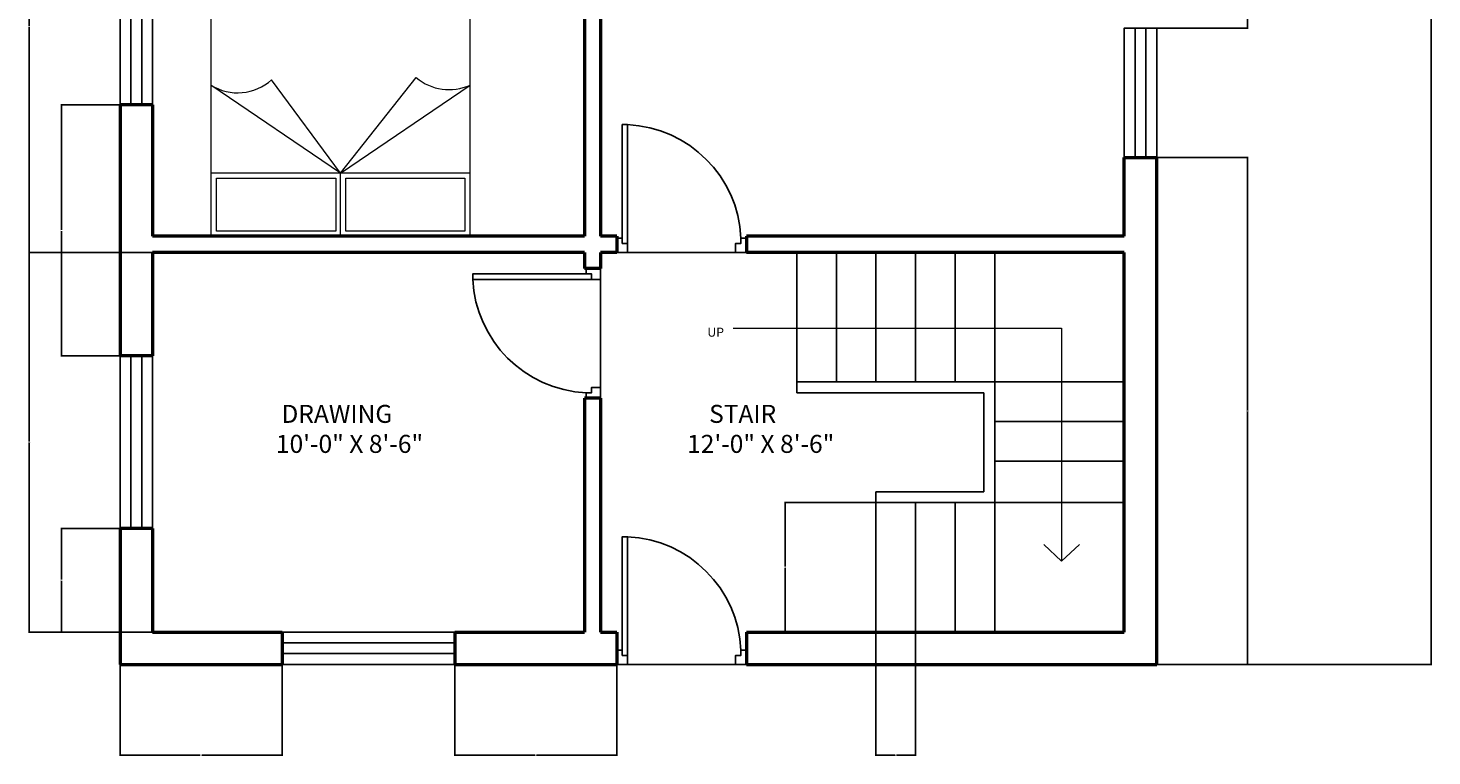
# Model space of a CAD drawing. Units: inches. Extents: x 17078 to 17468, y 5298 to 5853.
# Tile 1 of 3: x 17078 to 17468, y 5298 to 5500. Entities that reach past the tile are written whole.
import ezdxf

# ---------------------------------------------------------------- set-up
doc = ezdxf.new("R2010")
doc.units = ezdxf.units.IN
for name, color, linetype, lineweight in [('A-ANNO-DIMS', 2, 'Continuous', 18), ('A-ANNO-SYMB', 7, 'Continuous', 18), ('A-ANNO-TEXT', 7, 'Continuous', 18), ('A-AREA-IDEN', 7, 'Continuous', 18), ('door', 30, 'Continuous', 25), ('furniture', 9, 'Continuous', 18), ('Staircase', 11, 'Continuous', 25), ('wall', 7, 'Continuous', 50), ('window1', 151, 'Continuous', 25)]:
    doc.layers.add(name, color=color, linetype=linetype, lineweight=lineweight)
doc.styles.get("Standard").update_dxf_attribs({"font": 'arial.ttf'})
doc.dimstyles.get("Standard").update_dxf_attribs({"dimtxt": 0.18, "dimasz": 0.18, "dimexe": 0.18, "dimexo": 0.0625, "dimgap": 0.09, "dimtad": 0, "dimtih": 1, "dimtoh": 1, "dimdec": 4, "dimzin": 0, "dimdsep": 46, "dimtxsty": 'Standard', "dimcen": 0.09, "dimadec": 0, "dimazin": 0, "dimtfac": 1, "dimtdec": 4, "dimtofl": 0, "dimtmove": 0, "dimatfit": 3, "dimfxl": 1, "dimtolj": 1, "dimtzin": 0, "dimarcsym": 0})

# ---------------------------------------------------------------- blocks, each defined once
blk = doc.blocks.new('w2')
at = {"layer": 'window1'}
for p, q in [((17539.72, 5675.98), (17539.72, 5627.98)), ((17542.72, 5675.98), (17542.72, 5627.98))]:
    blk.add_line(p, q, dxfattribs=at)
blk.add_lwpolyline([(17536.72, 5627.98), (17545.72, 5627.98), (17545.72, 5675.98), (17536.72, 5675.98)], close=True, dxfattribs=at)
blk = doc.blocks.new('w1')
at = {"layer": 'window1'}
for p, q in [((17477.6, 5616.65), (17477.6, 5580.65)), ((17480.6, 5616.65), (17480.6, 5580.65))]:
    blk.add_line(p, q, dxfattribs=at)
blk.add_lwpolyline([(17474.6, 5580.65), (17483.6, 5580.65), (17483.6, 5616.65), (17474.6, 5616.65)], close=True, dxfattribs=at)
blk = doc.blocks.new('d1')
at = {"layer": 'door'}
blk.add_line((17631.7, 5593.67), (17667.7, 5593.67), dxfattribs=at)
blk.add_lwpolyline([(17633.2, 5596.17), (17634.7, 5596.17), (17634.7, 5629.17), (17633.2, 5629.17)], close=True, dxfattribs=at)
for points in [[(17634.7, 5593.67), (17631.7, 5593.67), (17631.7, 5597.67), (17633.2, 5597.67), (17633.2, 5596.17), (17634.7, 5596.17), (17634.7, 5593.67)], [(17664.7, 5593.67), (17667.7, 5593.67), (17667.7, 5597.67), (17666.2, 5597.67), (17666.2, 5596.17), (17664.7, 5596.17), (17664.7, 5593.67)]]:
    blk.add_lwpolyline(points, dxfattribs=at)
blk.add_arc((17633.2, 5596.17), 33.03, 2.6026, 87.3974, dxfattribs=at)
blk = doc.blocks.new('BED')
at = {"layer": 'furniture'}
for p, q in [((17631.72, 5825.16), (17631.72, 5807.64)), ((17595.72, 5807.64), (17667.72, 5807.64)), ((17631.72, 5807.64), (17595.72, 5783.16)), ((17631.72, 5807.64), (17610.71, 5781.09)), ((17631.72, 5807.64), (17667.72, 5783.16)), ((17631.72, 5807.64), (17650.87, 5781.67))]:
    blk.add_line(p, q, dxfattribs=at)
for points in [[(17595.72, 5741.16), (17667.72, 5741.16), (17667.72, 5825.16), (17595.72, 5825.16)], [(17597.14, 5823.74), (17630.27, 5823.74), (17630.27, 5809), (17597.14, 5809)], [(17633.01, 5823.74), (17666.14, 5823.74), (17666.14, 5809), (17633.01, 5809)]]:
    blk.add_lwpolyline(points, close=True, dxfattribs=at)
for centre, radius, start, end in [((17601.58, 5770.29), 14.15, 49.7949, 114.4561), ((17660.27, 5771.38), 13.94, 57.7012, 132.4176)]:
    blk.add_arc(centre, radius, start, end, dxfattribs=at)
blk = doc.blocks.new('*D22')
at = {"layer": 'A-ANNO-DIMS', "color": 0, "lineweight": -2, "transparency": 16777216}
for p, q in [((17391.6, 5827.52), (17467.96, 5827.52)), ((17467.78, 5827.34), (17467.78, 5575.7)), ((17467.78, 5323.7), (17467.78, 5575.34)), ((17391.6, 5323.52), (17467.96, 5323.52))]:
    blk.add_line(p, q, dxfattribs=at)
at = {"layer": 'A-ANNO-DIMS', "color": 0, "transparency": 16777216}
for points in [[(17467.75, 5827.34), (17467.81, 5827.34), (17467.78, 5827.52)], [(17467.75, 5323.7), (17467.81, 5323.7), (17467.78, 5323.52)]]:
    blk.add_solid(points, dxfattribs=at)
at = {"layer": 'Defpoints', "color": 0, "transparency": 16777216}
for p in [(17391.53, 5827.52), (17467.78, 5827.52), (17391.53, 5323.52)]:
    blk.add_point(p, dxfattribs=at)
at = {"layer": 'A-ANNO-DIMS', "color": 0, "transparency": 16777216, "insert": (17467.78, 5575.52), "char_height": 0.18, "attachment_point": 5}
blk.add_mtext('\\A1;504', dxfattribs=at)
blk = doc.blocks.new('*D23')
at = {"layer": 'A-ANNO-DIMS', "color": 0, "lineweight": -2, "transparency": 16777216}
for p, q in [((17112.47, 5438.02), (17078.1, 5438.02)), ((17078.28, 5437.84), (17078.28, 5385.45)), ((17078.28, 5332.7), (17078.28, 5385.09)), ((17112.47, 5332.52), (17078.1, 5332.52))]:
    blk.add_line(p, q, dxfattribs=at)
at = {"layer": 'A-ANNO-DIMS', "color": 0, "transparency": 16777216}
for points in [[(17078.25, 5437.84), (17078.31, 5437.84), (17078.28, 5438.02)], [(17078.25, 5332.7), (17078.31, 5332.7), (17078.28, 5332.52)]]:
    blk.add_solid(points, dxfattribs=at)
at = {"layer": 'Defpoints', "color": 0, "transparency": 16777216}
for p in [(17078.28, 5438.02), (17112.53, 5438.02), (17112.53, 5332.52)]:
    blk.add_point(p, dxfattribs=at)
at = {"layer": 'A-ANNO-DIMS', "color": 0, "transparency": 16777216, "insert": (17078.28, 5385.27), "char_height": 0.18, "attachment_point": 5}
blk.add_mtext('\\A1;105.5', dxfattribs=at)
blk = doc.blocks.new('*D24')
at = {"layer": 'A-ANNO-DIMS', "color": 0, "lineweight": -2, "transparency": 16777216}
for p, q in [((17112.47, 5563.52), (17078.1, 5563.52)), ((17078.28, 5563.34), (17078.28, 5500.95)), ((17078.28, 5438.2), (17078.28, 5500.59)), ((17112.47, 5438.02), (17078.1, 5438.02))]:
    blk.add_line(p, q, dxfattribs=at)
at = {"layer": 'A-ANNO-DIMS', "color": 0, "transparency": 16777216}
for points in [[(17078.25, 5563.34), (17078.31, 5563.34), (17078.28, 5563.52)], [(17078.25, 5438.2), (17078.31, 5438.2), (17078.28, 5438.02)]]:
    blk.add_solid(points, dxfattribs=at)
at = {"layer": 'Defpoints', "color": 0, "transparency": 16777216}
for p in [(17078.28, 5563.52), (17112.53, 5563.52), (17112.53, 5438.02)]:
    blk.add_point(p, dxfattribs=at)
at = {"layer": 'A-ANNO-DIMS', "color": 0, "transparency": 16777216, "insert": (17078.28, 5500.77), "char_height": 0.18, "attachment_point": 5}
blk.add_mtext('\\A1;125.5', dxfattribs=at)
blk = doc.blocks.new('*D26')
at = {"layer": 'A-ANNO-DIMS', "color": 0, "lineweight": -2, "transparency": 16777216}
for p, q in [((17103.53, 5323.46), (17103.53, 5298.09)), ((17148.53, 5323.46), (17148.53, 5298.09)), ((17103.71, 5298.27), (17125.81, 5298.27)), ((17148.35, 5298.27), (17126.26, 5298.27))]:
    blk.add_line(p, q, dxfattribs=at)
at = {"layer": 'A-ANNO-DIMS', "color": 0, "transparency": 16777216}
for points in [[(17103.71, 5298.3), (17103.71, 5298.24), (17103.53, 5298.27)], [(17148.35, 5298.3), (17148.35, 5298.24), (17148.53, 5298.27)]]:
    blk.add_solid(points, dxfattribs=at)
at = {"layer": 'Defpoints', "color": 0, "transparency": 16777216}
for p in [(17103.53, 5323.52), (17148.53, 5323.52), (17148.53, 5298.27)]:
    blk.add_point(p, dxfattribs=at)
at = {"layer": 'A-ANNO-DIMS', "color": 0, "transparency": 16777216, "insert": (17126.03, 5298.27), "char_height": 0.18, "attachment_point": 5}
blk.add_mtext('\\A1;45', dxfattribs=at)
blk = doc.blocks.new('*D27')
at = {"layer": 'A-ANNO-DIMS', "color": 0, "lineweight": -2, "transparency": 16777216}
for p, q in [((17196.53, 5323.46), (17196.53, 5298.09)), ((17241.53, 5323.46), (17241.53, 5298.09)), ((17196.71, 5298.27), (17218.81, 5298.27)), ((17241.35, 5298.27), (17219.26, 5298.27))]:
    blk.add_line(p, q, dxfattribs=at)
at = {"layer": 'A-ANNO-DIMS', "color": 0, "transparency": 16777216}
for points in [[(17196.71, 5298.3), (17196.71, 5298.24), (17196.53, 5298.27)], [(17241.35, 5298.3), (17241.35, 5298.24), (17241.53, 5298.27)]]:
    blk.add_solid(points, dxfattribs=at)
at = {"layer": 'Defpoints', "color": 0, "transparency": 16777216}
for p in [(17196.53, 5323.52), (17241.53, 5323.52), (17241.53, 5298.27)]:
    blk.add_point(p, dxfattribs=at)
at = {"layer": 'A-ANNO-DIMS', "color": 0, "transparency": 16777216, "insert": (17219.03, 5298.27), "char_height": 0.18, "attachment_point": 5}
blk.add_mtext('\\A1;45', dxfattribs=at)
blk = doc.blocks.new('*D28')
at = {"layer": 'A-ANNO-DIMS', "color": 0, "lineweight": -2, "transparency": 16777216}
for p, q in [((17112.47, 5361.27), (17087.1, 5361.27)), ((17087.28, 5361.09), (17087.28, 5347.08)), ((17087.28, 5332.7), (17087.28, 5346.71)), ((17112.47, 5332.52), (17087.1, 5332.52))]:
    blk.add_line(p, q, dxfattribs=at)
at = {"layer": 'A-ANNO-DIMS', "color": 0, "transparency": 16777216}
for points in [[(17087.25, 5361.09), (17087.31, 5361.09), (17087.28, 5361.27)], [(17087.25, 5332.7), (17087.31, 5332.7), (17087.28, 5332.52)]]:
    blk.add_solid(points, dxfattribs=at)
at = {"layer": 'Defpoints', "color": 0, "transparency": 16777216}
for p in [(17087.28, 5361.27), (17112.53, 5361.27), (17112.53, 5332.52)]:
    blk.add_point(p, dxfattribs=at)
at = {"layer": 'A-ANNO-DIMS', "color": 0, "transparency": 16777216, "insert": (17087.28, 5346.9), "char_height": 0.18, "attachment_point": 5}
blk.add_mtext('\\A1;28.75', dxfattribs=at)
blk = doc.blocks.new('*D29')
at = {"layer": 'A-ANNO-DIMS', "color": 0, "lineweight": -2, "transparency": 16777216}
for p, q in [((17112.47, 5479.02), (17087.1, 5479.02)), ((17087.28, 5478.84), (17087.28, 5444.33)), ((17087.28, 5409.45), (17087.28, 5443.96)), ((17112.47, 5409.27), (17087.1, 5409.27))]:
    blk.add_line(p, q, dxfattribs=at)
at = {"layer": 'A-ANNO-DIMS', "color": 0, "transparency": 16777216}
for points in [[(17087.25, 5478.84), (17087.31, 5478.84), (17087.28, 5479.02)], [(17087.25, 5409.45), (17087.31, 5409.45), (17087.28, 5409.27)]]:
    blk.add_solid(points, dxfattribs=at)
at = {"layer": 'Defpoints', "color": 0, "transparency": 16777216}
for p in [(17087.28, 5479.02), (17112.53, 5479.02), (17112.53, 5409.27)]:
    blk.add_point(p, dxfattribs=at)
at = {"layer": 'A-ANNO-DIMS', "color": 0, "transparency": 16777216, "insert": (17087.28, 5444.15), "char_height": 0.18, "attachment_point": 5}
blk.add_mtext('\\A1;69.75', dxfattribs=at)
blk = doc.blocks.new('*D32')
at = {"layer": 'A-ANNO-DIMS', "color": 0, "lineweight": -2, "transparency": 16777216}
for p, q in [((17391.6, 5464.35), (17416.96, 5464.35)), ((17416.78, 5464.17), (17416.78, 5394.12)), ((17416.78, 5323.7), (17416.78, 5393.76)), ((17391.6, 5323.52), (17416.96, 5323.52))]:
    blk.add_line(p, q, dxfattribs=at)
at = {"layer": 'A-ANNO-DIMS', "color": 0, "transparency": 16777216}
for points in [[(17416.75, 5464.17), (17416.81, 5464.17), (17416.78, 5464.35)], [(17416.75, 5323.7), (17416.81, 5323.7), (17416.78, 5323.52)]]:
    blk.add_solid(points, dxfattribs=at)
at = {"layer": 'Defpoints', "color": 0, "transparency": 16777216}
for p in [(17391.53, 5464.35), (17391.53, 5323.52), (17416.78, 5323.52)]:
    blk.add_point(p, dxfattribs=at)
at = {"layer": 'A-ANNO-DIMS', "color": 0, "transparency": 16777216, "insert": (17416.78, 5393.94), "char_height": 0.18, "attachment_point": 5}
blk.add_mtext('\\A1;140.83', dxfattribs=at)
blk = doc.blocks.new('*D33')
at = {"layer": 'A-ANNO-DIMS', "color": 0, "lineweight": -2, "transparency": 16777216}
for p, q in [((17391.6, 5544.03), (17416.96, 5544.03)), ((17416.78, 5543.85), (17416.78, 5522.37)), ((17416.78, 5500.53), (17416.78, 5522.01)), ((17391.6, 5500.35), (17416.96, 5500.35))]:
    blk.add_line(p, q, dxfattribs=at)
at = {"layer": 'A-ANNO-DIMS', "color": 0, "transparency": 16777216}
for points in [[(17416.75, 5543.85), (17416.81, 5543.85), (17416.78, 5544.03)], [(17416.75, 5500.53), (17416.81, 5500.53), (17416.78, 5500.35)]]:
    blk.add_solid(points, dxfattribs=at)
at = {"layer": 'Defpoints', "color": 0, "transparency": 16777216}
for p in [(17391.53, 5544.03), (17391.53, 5500.35), (17416.78, 5500.35)]:
    blk.add_point(p, dxfattribs=at)
at = {"layer": 'A-ANNO-DIMS', "color": 0, "transparency": 16777216, "insert": (17416.78, 5522.19), "char_height": 0.18, "attachment_point": 5}
blk.add_mtext('\\A1;43.67', dxfattribs=at)
blk = doc.blocks.new('*D40')
at = {"layer": 'A-ANNO-DIMS', "color": 0, "lineweight": -2, "transparency": 16777216}
for p, q in [((17313.47, 5368.52), (17288.1, 5368.52)), ((17288.28, 5368.34), (17288.28, 5350.7)), ((17288.28, 5332.7), (17288.28, 5350.34)), ((17313.47, 5332.52), (17288.1, 5332.52))]:
    blk.add_line(p, q, dxfattribs=at)
at = {"layer": 'A-ANNO-DIMS', "color": 0, "transparency": 16777216}
for points in [[(17288.25, 5368.34), (17288.31, 5368.34), (17288.28, 5368.52)], [(17288.25, 5332.7), (17288.31, 5332.7), (17288.28, 5332.52)]]:
    blk.add_solid(points, dxfattribs=at)
at = {"layer": 'Defpoints', "color": 0, "transparency": 16777216}
for p in [(17288.28, 5368.52), (17313.53, 5368.52), (17313.53, 5332.52)]:
    blk.add_point(p, dxfattribs=at)
at = {"layer": 'A-ANNO-DIMS', "color": 0, "transparency": 16777216, "insert": (17288.28, 5350.52), "char_height": 0.18, "attachment_point": 5}
blk.add_mtext('\\A1;36', dxfattribs=at)
blk = doc.blocks.new('*D41')
at = {"layer": 'A-ANNO-DIMS', "color": 0, "lineweight": -2, "transparency": 16777216}
for p, q in [((17313.53, 5332.46), (17313.53, 5298.09)), ((17324.53, 5332.46), (17324.53, 5298.09)), ((17313.71, 5298.27), (17318.84, 5298.27)), ((17324.35, 5298.27), (17319.23, 5298.27))]:
    blk.add_line(p, q, dxfattribs=at)
at = {"layer": 'A-ANNO-DIMS', "color": 0, "transparency": 16777216}
for points in [[(17313.71, 5298.3), (17313.71, 5298.24), (17313.53, 5298.27)], [(17324.35, 5298.3), (17324.35, 5298.24), (17324.53, 5298.27)]]:
    blk.add_solid(points, dxfattribs=at)
at = {"layer": 'Defpoints', "color": 0, "transparency": 16777216}
for p in [(17313.53, 5332.52), (17324.53, 5332.52), (17324.53, 5298.27)]:
    blk.add_point(p, dxfattribs=at)
at = {"layer": 'A-ANNO-DIMS', "color": 0, "transparency": 16777216, "insert": (17319.03, 5298.27), "char_height": 0.18, "attachment_point": 5}
blk.add_mtext('\\A1;11', dxfattribs=at)

msp = doc.modelspace()

# ---------------------------------------------------------------- linework, layer by layer
at = {"layer": 'A-ANNO-SYMB'}
for p, q in [((17273.8519, 5416.9969), (17365.0944, 5416.9969)), ((17365.0944, 5416.9969), (17365.0944, 5352.2347)), ((17365.0944, 5352.2347), (17360.133, 5356.8275)), ((17365.0944, 5352.2347), (17370.0557, 5356.8275))]:
    msp.add_line(p, q, dxfattribs=at)
at = {"layer": 'Staircase'}
for p, q in [((17291.534, 5402.02), (17291.534, 5438.02)), ((17302.534, 5402.02), (17302.534, 5438.02)), ((17313.534, 5402.02), (17313.534, 5438.02)), ((17324.534, 5402.02), (17324.534, 5438.02)), ((17335.534, 5402.02), (17335.534, 5438.02)), ((17346.534, 5332.52), (17346.534, 5438.02)), ((17382.534, 5402.02), (17291.534, 5402.02)), ((17291.534, 5402.02), (17291.534, 5399.02)), ((17343.534, 5399.02), (17291.534, 5399.02)), ((17343.534, 5371.52), (17343.534, 5399.02)), ((17382.534, 5391.02), (17346.534, 5391.02)), ((17382.534, 5380.02), (17346.534, 5380.02)), ((17313.534, 5371.52), (17343.534, 5371.52)), ((17313.534, 5371.52), (17313.534, 5368.52)), ((17313.534, 5332.52), (17313.534, 5368.52)), ((17313.534, 5368.52), (17382.534, 5368.52)), ((17324.534, 5332.52), (17324.534, 5368.52)), ((17335.534, 5332.52), (17335.534, 5368.52))]:
    msp.add_line(p, q, dxfattribs=at)
at = {"layer": 'wall'}
for p, q in [((17237.034, 5568.02), (17237.034, 5442.52)), ((17232.534, 5563.52), (17232.534, 5442.52)), ((17112.534, 5479.02), (17103.534, 5479.02)), ((17103.534, 5479.02), (17103.534, 5409.27)), ((17112.534, 5479.02), (17112.534, 5442.52)), ((17382.534, 5442.52), (17382.534, 5464.3549)), ((17382.534, 5464.3549), (17391.534, 5464.3549)), ((17391.534, 5323.52), (17391.534, 5464.3549)), ((17232.534, 5442.52), (17112.534, 5442.52)), ((17241.534, 5442.52), (17237.034, 5442.52)), ((17241.534, 5442.52), (17241.534, 5438.02)), ((17382.534, 5442.52), (17277.534, 5442.52)), ((17277.534, 5442.52), (17277.534, 5438.02)), ((17112.534, 5438.02), (17112.534, 5409.27)), ((17232.534, 5438.02), (17112.534, 5438.02)), ((17232.534, 5438.02), (17232.534, 5433.52)), ((17237.034, 5438.02), (17237.034, 5433.52)), ((17241.534, 5438.02), (17237.034, 5438.02)), ((17382.534, 5438.02), (17277.534, 5438.02)), ((17382.534, 5332.52), (17382.534, 5438.02)), ((17237.034, 5433.52), (17232.534, 5433.52)), ((17112.534, 5409.27), (17103.534, 5409.27)), ((17237.034, 5397.52), (17232.534, 5397.52)), ((17232.534, 5397.52), (17232.534, 5332.52)), ((17237.034, 5397.52), (17237.034, 5332.52)), ((17112.534, 5361.27), (17103.534, 5361.27)), ((17103.534, 5361.27), (17103.534, 5323.52)), ((17112.534, 5361.27), (17112.534, 5332.52)), ((17112.534, 5332.52), (17148.534, 5332.52)), ((17148.534, 5332.52), (17148.534, 5323.52)), ((17196.534, 5332.52), (17196.534, 5323.52)), ((17196.534, 5332.52), (17232.534, 5332.52)), ((17237.034, 5332.52), (17241.534, 5332.52)), ((17241.534, 5332.52), (17241.534, 5323.52)), ((17277.534, 5332.52), (17277.534, 5323.52)), ((17277.534, 5332.52), (17382.534, 5332.52)), ((17103.534, 5323.52), (17148.534, 5323.52)), ((17196.534, 5323.52), (17241.534, 5323.52)), ((17277.534, 5323.52), (17391.534, 5323.52))]:
    msp.add_line(p, q, dxfattribs=at)

# ---------------------------------------------------------------- block references
at = {"layer": 'door'}
for p in [(-390.1629, -155.6529), (-390.1629, -270.1529)]:
    msp.add_blockref('d1', p, dxfattribs=at)
at = {"layer": 'door', "xscale": -1, "rotation": 90}
msp.add_blockref('d1', (22830.7069, 23065.2169), dxfattribs=at)
at = {"layer": 'furniture', "rotation": 180}
msp.add_blockref('BED', (34796.4989, 11267.683), dxfattribs=at)
at = {"layer": 'window1'}
for name, p in [('w2', (-433.1828, -148.959)), ('w1', (-92.0702, -116.2984)), ('w2', (-433.1828, -266.709))]:
    msp.add_blockref(name, p, dxfattribs=at)
at = {"layer": 'window1', "rotation": 270}
msp.add_blockref('w2', (11520.555, 22869.2368), dxfattribs=at)

# ---------------------------------------------------------------- texts
at = {"layer": 'A-ANNO-TEXT', "insert": (17266.6924, 5417.0862), "char_height": 2.5, "attachment_point": 1}
msp.add_mtext_dynamic_manual_height_columns('UP', width=14.245154, gutter_width=12.5, heights=[0], dxfattribs=at)
at = {"layer": 'A-AREA-IDEN', "char_height": 5, "attachment_point": 1}
for s, insert in [(' DRAWING \\P10\'-0" X 8\'-6"', (17146.8369, 5395.6419)), ('    STAIR\\P12\'-0" X 8\'-6"', (17261.0729, 5395.6419))]:
    msp.add_mtext_dynamic_manual_height_columns(s, width=48.964, gutter_width=12.5, heights=[0], dxfattribs=dict(at, insert=insert))

# ---------------------------------------------------------------- dimensions: what is measured, and where the dimension line sits
at = {"layer": 'A-ANNO-DIMS'}
for base, p1, p2, angle, override, picture, middle in [((17467.784, 5827.52), (17391.534, 5323.52), (17391.534, 5827.52), 90, {"dimdec": 0, "dimlfac": 1, "dimrnd": 0, "dimzin": 0, "dimdsep": 46, "dimlunit": 2}, '*D22', (17467.784, 5575.52)), ((17078.284, 5563.52), (17112.534, 5438.02), (17112.534, 5563.52), 90, {"dimdec": 1, "dimlfac": 1, "dimrnd": 0, "dimzin": 0, "dimdsep": 46, "dimlunit": 2}, '*D24', (17078.284, 5500.77)), ((17416.784, 5500.3549), (17391.534, 5544.0271), (17391.534, 5500.3549), 270, {"dimdec": 2, "dimlfac": 1, "dimrnd": 0, "dimzin": 0, "dimdsep": 46, "dimlunit": 2}, '*D33', (17416.784, 5522.191)), ((17087.284, 5479.02), (17112.534, 5409.27), (17112.534, 5479.02), 90, {"dimdec": 2, "dimlfac": 1, "dimrnd": 0, "dimzin": 0, "dimdsep": 46, "dimlunit": 2}, '*D29', (17087.284, 5444.145)), ((17416.784, 5323.52), (17391.534, 5464.3549), (17391.534, 5323.52), 270, {"dimdec": 2, "dimlfac": 1, "dimrnd": 0, "dimzin": 0, "dimdsep": 46, "dimlunit": 2}, '*D32', (17416.784, 5393.9374)), ((17078.284, 5438.02), (17112.534, 5332.52), (17112.534, 5438.02), 90, {"dimdec": 1, "dimlfac": 1, "dimrnd": 0, "dimzin": 0, "dimdsep": 46, "dimlunit": 2}, '*D23', (17078.284, 5385.27)), ((17288.284, 5368.52), (17313.534, 5332.52), (17313.534, 5368.52), 90, {"dimdec": 0, "dimlfac": 1, "dimrnd": 0, "dimzin": 0, "dimdsep": 46, "dimlunit": 2}, '*D40', (17288.284, 5350.52)), ((17087.284, 5361.27), (17112.534, 5332.52), (17112.534, 5361.27), 90, {"dimdec": 2, "dimlfac": 1, "dimrnd": 0, "dimzin": 0, "dimdsep": 46, "dimlunit": 2}, '*D28', (17087.284, 5346.895))]:
    dim = msp.add_linear_dim(base=base, p1=p1, p2=p2, angle=angle, dimstyle='Standard', override=override, dxfattribs=at)
    dim.commit()
    dim.dimension.update_dxf_attribs({"geometry": picture, "text_midpoint": middle})
for base, p1, p2, picture, middle in [((17324.534, 5298.27), (17313.534, 5332.52), (17324.534, 5332.52), '*D41', (17319.034, 5298.27)), ((17148.534, 5298.27), (17103.534, 5323.52), (17148.534, 5323.52), '*D26', (17126.034, 5298.27)), ((17241.534, 5298.27), (17196.534, 5323.52), (17241.534, 5323.52), '*D27', (17219.034, 5298.27))]:
    dim = msp.add_linear_dim(base=base, p1=p1, p2=p2, dimstyle='Standard', override={"dimdec": 0, "dimlfac": 1, "dimrnd": 0, "dimzin": 0, "dimdsep": 46, "dimlunit": 2}, dxfattribs=at)
    dim.commit()
    dim.dimension.update_dxf_attribs({"geometry": picture, "text_midpoint": middle})

doc.saveas('drawing.dxf')
